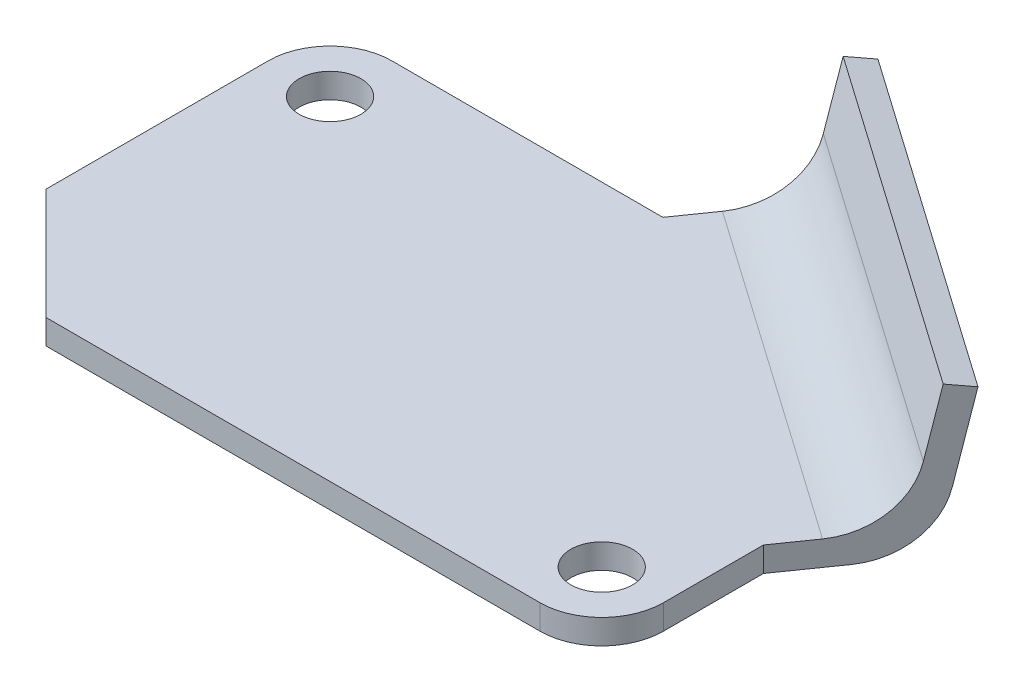
ISO-10303-21;
HEADER;
FILE_DESCRIPTION(('STEP AP214'),'2;1');
FILE_NAME('part.step','',(''),(''),'','','');
FILE_SCHEMA(('AUTOMOTIVE_DESIGN { 1 0 10303 214 1 1 1 1 }'));
ENDSEC;
DATA;
#1=APPLICATION_CONTEXT('core data for automotive mechanical design processes');
#2=APPLICATION_PROTOCOL_DEFINITION('international standard','automotive_design',2000,#1);
#3=PRODUCT_CONTEXT('',#1,'mechanical');
#4=PRODUCT('Part','Part','',(#3));
#5=PRODUCT_RELATED_PRODUCT_CATEGORY('part','',(#4));
#6=PRODUCT_DEFINITION_FORMATION('','',#4);
#7=PRODUCT_DEFINITION_CONTEXT('part definition',#1,'design');
#8=PRODUCT_DEFINITION('design','',#6,#7);
#9=PRODUCT_DEFINITION_SHAPE('','',#8);
#10=(LENGTH_UNIT() NAMED_UNIT(*) SI_UNIT(.MILLI.,.METRE.));
#11=(NAMED_UNIT(*) PLANE_ANGLE_UNIT() SI_UNIT($,.RADIAN.));
#12=(NAMED_UNIT(*) SI_UNIT($,.STERADIAN.) SOLID_ANGLE_UNIT());
#13=UNCERTAINTY_MEASURE_WITH_UNIT(LENGTH_MEASURE(1.E-05),#10,'distance_accuracy_value','');
#14=(GEOMETRIC_REPRESENTATION_CONTEXT(3) GLOBAL_UNCERTAINTY_ASSIGNED_CONTEXT((#13)) GLOBAL_UNIT_ASSIGNED_CONTEXT((#10,
#11,#12)) REPRESENTATION_CONTEXT('',''));
#15=CARTESIAN_POINT('',(0.,0.,0.));
#16=DIRECTION('',(0.,0.,1.));
#17=DIRECTION('',(1.,0.,0.));
#18=AXIS2_PLACEMENT_3D('',#15,#16,#17);
#19=CARTESIAN_POINT('',(0.,4.,-32.));
#20=DIRECTION('',(0.,0.,-1.));
#21=DIRECTION('',(-1.,0.,0.));
#22=AXIS2_PLACEMENT_3D('',#19,#20,#21);
#23=PLANE('',#22);
#24=DIRECTION('',(1.,0.,0.));
#25=VECTOR('',#24,1.);
#26=CARTESIAN_POINT('',(0.,0.,-32.));
#27=LINE('',#26,#25);
#28=CARTESIAN_POINT('',(-44.,0.,-32.));
#29=VERTEX_POINT('',#28);
#30=CARTESIAN_POINT('',(-0.0954306437080214,0.,-32.));
#31=VERTEX_POINT('',#30);
#32=EDGE_CURVE('E152',#29,#31,#27,.T.);
#33=ORIENTED_EDGE('',*,*,#32,.F.);
#34=DIRECTION('',(0.,-1.,0.));
#35=VECTOR('',#34,1.);
#36=CARTESIAN_POINT('',(-44.,4.,-32.));
#37=LINE('',#36,#35);
#38=CARTESIAN_POINT('',(-44.,4.,-32.));
#39=VERTEX_POINT('',#38);
#40=EDGE_CURVE('E241',#29,#39,#37,.F.);
#41=ORIENTED_EDGE('',*,*,#40,.T.);
#42=DIRECTION('',(1.,0.,0.));
#43=VECTOR('',#42,1.);
#44=CARTESIAN_POINT('',(0.,4.,-32.));
#45=LINE('',#44,#43);
#46=CARTESIAN_POINT('',(-0.0954306437080214,4.,-32.));
#47=VERTEX_POINT('',#46);
#48=EDGE_CURVE('E224',#39,#47,#45,.T.);
#49=ORIENTED_EDGE('',*,*,#48,.T.);
#50=DIRECTION('',(0.,-1.,0.));
#51=VECTOR('',#50,1.);
#52=CARTESIAN_POINT('',(-0.0954306437080294,4.,-32.));
#53=LINE('',#52,#51);
#54=EDGE_CURVE('E204',#47,#31,#53,.T.);
#55=ORIENTED_EDGE('',*,*,#54,.T.);
#56=EDGE_LOOP('',(#33,#41,#49,#55));
#57=FACE_BOUND('',#56,.T.);
#58=ADVANCED_FACE('F43',(#57),#23,.T.);
#59=CARTESIAN_POINT('',(0.,4.,0.));
#60=DIRECTION('',(0.,1.,0.));
#61=DIRECTION('',(0.,0.,1.));
#62=AXIS2_PLACEMENT_3D('',#59,#60,#61);
#63=PLANE('',#62);
#64=CARTESIAN_POINT('',(-44.,4.,-22.));
#65=DIRECTION('',(0.,1.,0.));
#66=DIRECTION('',(0.,0.,1.));
#67=AXIS2_PLACEMENT_3D('',#64,#65,#66);
#68=CIRCLE('',#67,5.);
#69=CARTESIAN_POINT('',(-44.,4.,-17.));
#70=VERTEX_POINT('',#69);
#71=EDGE_CURVE('E258',#70,#70,#68,.T.);
#72=ORIENTED_EDGE('',*,*,#71,.F.);
#73=EDGE_LOOP('',(#72));
#74=FACE_BOUND('',#73,.T.);
#75=CARTESIAN_POINT('',(44.,4.,22.));
#76=DIRECTION('',(0.,1.,0.));
#77=DIRECTION('',(0.,0.,1.));
#78=AXIS2_PLACEMENT_3D('',#75,#76,#77);
#79=CIRCLE('',#78,5.);
#80=CARTESIAN_POINT('',(44.,4.,27.));
#81=VERTEX_POINT('',#80);
#82=EDGE_CURVE('E263',#81,#81,#79,.T.);
#83=ORIENTED_EDGE('',*,*,#82,.F.);
#84=EDGE_LOOP('',(#83));
#85=FACE_BOUND('',#84,.T.);
#86=DIRECTION('',(0.,0.,-1.));
#87=VECTOR('',#86,1.);
#88=CARTESIAN_POINT('',(-54.,4.,0.));
#89=LINE('',#88,#87);
#90=CARTESIAN_POINT('',(-54.,4.,13.9999999999999));
#91=VERTEX_POINT('',#90);
#92=CARTESIAN_POINT('',(-54.,4.,-22.));
#93=VERTEX_POINT('',#92);
#94=EDGE_CURVE('E225',#91,#93,#89,.T.);
#95=ORIENTED_EDGE('',*,*,#94,.F.);
#96=DIRECTION('',(0.707106781186548,0.,0.707106781186548));
#97=VECTOR('',#96,1.);
#98=CARTESIAN_POINT('',(-34.,4.,34.));
#99=LINE('',#98,#97);
#100=CARTESIAN_POINT('',(-35.9999999999999,4.,32.));
#101=VERTEX_POINT('',#100);
#102=EDGE_CURVE('E11',#91,#101,#99,.T.);
#103=ORIENTED_EDGE('',*,*,#102,.T.);
#104=DIRECTION('',(1.,0.,0.));
#105=VECTOR('',#104,1.);
#106=CARTESIAN_POINT('',(0.,4.,32.));
#107=LINE('',#106,#105);
#108=CARTESIAN_POINT('',(44.,4.,32.));
#109=VERTEX_POINT('',#108);
#110=EDGE_CURVE('E217',#101,#109,#107,.T.);
#111=ORIENTED_EDGE('',*,*,#110,.T.);
#112=CARTESIAN_POINT('',(44.,4.,22.));
#113=DIRECTION('',(0.,1.,0.));
#114=DIRECTION('',(0.,0.,1.));
#115=AXIS2_PLACEMENT_3D('',#112,#113,#114);
#116=CIRCLE('',#115,10.);
#117=CARTESIAN_POINT('',(54.,4.,22.));
#118=VERTEX_POINT('',#117);
#119=EDGE_CURVE('E243',#109,#118,#116,.T.);
#120=ORIENTED_EDGE('',*,*,#119,.T.);
#121=DIRECTION('',(0.,0.,-1.));
#122=VECTOR('',#121,1.);
#123=CARTESIAN_POINT('',(54.,4.,0.));
#124=LINE('',#123,#122);
#125=CARTESIAN_POINT('',(54.,4.,5.81120706332445));
#126=VERTEX_POINT('',#125);
#127=EDGE_CURVE('E220',#118,#126,#124,.T.);
#128=ORIENTED_EDGE('',*,*,#127,.T.);
#129=DIRECTION('',(-0.573576436351047,0.,0.819152044288991));
#130=VECTOR('',#129,1.);
#131=CARTESIAN_POINT('',(59.7357643635105,4.,-2.38031337956546));
#132=LINE('',#131,#130);
#133=CARTESIAN_POINT('',(57.9434998164939,4.,0.17930566081089));
#134=VERTEX_POINT('',#133);
#135=EDGE_CURVE('E208',#134,#126,#132,.T.);
#136=ORIENTED_EDGE('',*,*,#135,.F.);
#137=DIRECTION('',(0.819152044288991,0.,0.573576436351048));
#138=VECTOR('',#137,1.);
#139=CARTESIAN_POINT('',(3.87946489342047,4.,-37.6767391383582));
#140=LINE('',#139,#138);
#141=CARTESIAN_POINT('',(3.87946489342047,4.,-37.6767391383582));
#142=VERTEX_POINT('',#141);
#143=EDGE_CURVE('E196',#142,#134,#140,.T.);
#144=ORIENTED_EDGE('',*,*,#143,.F.);
#145=DIRECTION('',(-0.573576436351048,0.,0.819152044288991));
#146=VECTOR('',#145,1.);
#147=CARTESIAN_POINT('',(-1.49365590296264,4.,-30.0031273830191));
#148=LINE('',#147,#146);
#149=EDGE_CURVE('E164',#142,#47,#148,.T.);
#150=ORIENTED_EDGE('',*,*,#149,.T.);
#151=ORIENTED_EDGE('',*,*,#48,.F.);
#152=CARTESIAN_POINT('',(-44.,4.,-22.));
#153=DIRECTION('',(0.,1.,0.));
#154=DIRECTION('',(0.,0.,1.));
#155=AXIS2_PLACEMENT_3D('',#152,#153,#154);
#156=CIRCLE('',#155,10.);
#157=EDGE_CURVE('E244',#39,#93,#156,.T.);
#158=ORIENTED_EDGE('',*,*,#157,.T.);
#159=EDGE_LOOP('',(#95,#103,#111,#120,#128,#136,#144,#150,#151,#158));
#160=FACE_BOUND('',#159,.T.);
#161=ADVANCED_FACE('F273',(#74,#85,#160),#63,.T.);
#162=CARTESIAN_POINT('',(0.,4.,32.));
#163=DIRECTION('',(0.,0.,-1.));
#164=DIRECTION('',(-1.,0.,0.));
#165=AXIS2_PLACEMENT_3D('',#162,#163,#164);
#166=PLANE('',#165);
#167=ORIENTED_EDGE('',*,*,#110,.F.);
#168=DIRECTION('',(0.,-1.,0.));
#169=VECTOR('',#168,1.);
#170=CARTESIAN_POINT('',(-35.9999999999999,0.,32.));
#171=LINE('',#170,#169);
#172=CARTESIAN_POINT('',(-35.9999999999999,0.,32.));
#173=VERTEX_POINT('',#172);
#174=EDGE_CURVE('E251',#101,#173,#171,.T.);
#175=ORIENTED_EDGE('',*,*,#174,.T.);
#176=DIRECTION('',(1.,0.,0.));
#177=VECTOR('',#176,1.);
#178=CARTESIAN_POINT('',(0.,0.,32.));
#179=LINE('',#178,#177);
#180=CARTESIAN_POINT('',(44.,0.,32.));
#181=VERTEX_POINT('',#180);
#182=EDGE_CURVE('E213',#173,#181,#179,.T.);
#183=ORIENTED_EDGE('',*,*,#182,.T.);
#184=DIRECTION('',(0.,-1.,0.));
#185=VECTOR('',#184,1.);
#186=CARTESIAN_POINT('',(44.,4.,32.));
#187=LINE('',#186,#185);
#188=EDGE_CURVE('E252',#181,#109,#187,.F.);
#189=ORIENTED_EDGE('',*,*,#188,.T.);
#190=EDGE_LOOP('',(#167,#175,#183,#189));
#191=FACE_BOUND('',#190,.T.);
#192=ADVANCED_FACE('F279',(#191),#166,.F.);
#193=CARTESIAN_POINT('',(54.,4.,0.));
#194=DIRECTION('',(-1.,0.,0.));
#195=DIRECTION('',(0.,0.,1.));
#196=AXIS2_PLACEMENT_3D('',#193,#194,#195);
#197=PLANE('',#196);
#198=ORIENTED_EDGE('',*,*,#127,.F.);
#199=DIRECTION('',(0.,-1.,0.));
#200=VECTOR('',#199,1.);
#201=CARTESIAN_POINT('',(54.,4.,22.));
#202=LINE('',#201,#200);
#203=CARTESIAN_POINT('',(54.,0.,22.));
#204=VERTEX_POINT('',#203);
#205=EDGE_CURVE('E247',#118,#204,#202,.T.);
#206=ORIENTED_EDGE('',*,*,#205,.T.);
#207=DIRECTION('',(0.,0.,-1.));
#208=VECTOR('',#207,1.);
#209=CARTESIAN_POINT('',(54.,0.,0.));
#210=LINE('',#209,#208);
#211=CARTESIAN_POINT('',(54.,0.,5.81120706332445));
#212=VERTEX_POINT('',#211);
#213=EDGE_CURVE('E227',#204,#212,#210,.T.);
#214=ORIENTED_EDGE('',*,*,#213,.T.);
#215=DIRECTION('',(0.,-1.,0.));
#216=VECTOR('',#215,1.);
#217=CARTESIAN_POINT('',(54.,4.,5.81120706332445));
#218=LINE('',#217,#216);
#219=EDGE_CURVE('E222',#126,#212,#218,.T.);
#220=ORIENTED_EDGE('',*,*,#219,.F.);
#221=EDGE_LOOP('',(#198,#206,#214,#220));
#222=FACE_BOUND('',#221,.T.);
#223=ADVANCED_FACE('F299',(#222),#197,.F.);
#224=CARTESIAN_POINT('',(-54.,4.,0.));
#225=DIRECTION('',(-1.,0.,0.));
#226=DIRECTION('',(0.,0.,1.));
#227=AXIS2_PLACEMENT_3D('',#224,#225,#226);
#228=PLANE('',#227);
#229=DIRECTION('',(0.,0.,-1.));
#230=VECTOR('',#229,1.);
#231=CARTESIAN_POINT('',(-54.,0.,0.));
#232=LINE('',#231,#230);
#233=CARTESIAN_POINT('',(-54.,0.,13.9999999999999));
#234=VERTEX_POINT('',#233);
#235=CARTESIAN_POINT('',(-54.,0.,-22.));
#236=VERTEX_POINT('',#235);
#237=EDGE_CURVE('E216',#234,#236,#232,.T.);
#238=ORIENTED_EDGE('',*,*,#237,.F.);
#239=DIRECTION('',(0.,1.,0.));
#240=VECTOR('',#239,1.);
#241=CARTESIAN_POINT('',(-54.,4.,13.9999999999999));
#242=LINE('',#241,#240);
#243=EDGE_CURVE('E52',#234,#91,#242,.T.);
#244=ORIENTED_EDGE('',*,*,#243,.T.);
#245=ORIENTED_EDGE('',*,*,#94,.T.);
#246=DIRECTION('',(0.,-1.,0.));
#247=VECTOR('',#246,1.);
#248=CARTESIAN_POINT('',(-54.,4.,-22.));
#249=LINE('',#248,#247);
#250=EDGE_CURVE('E231',#93,#236,#249,.T.);
#251=ORIENTED_EDGE('',*,*,#250,.T.);
#252=EDGE_LOOP('',(#238,#244,#245,#251));
#253=FACE_BOUND('',#252,.T.);
#254=ADVANCED_FACE('F312',(#253),#228,.T.);
#255=CARTESIAN_POINT('',(0.,0.,0.));
#256=DIRECTION('',(0.,1.,0.));
#257=DIRECTION('',(0.,0.,1.));
#258=AXIS2_PLACEMENT_3D('',#255,#256,#257);
#259=PLANE('',#258);
#260=CARTESIAN_POINT('',(-44.,0.,-22.));
#261=DIRECTION('',(0.,1.,0.));
#262=DIRECTION('',(0.,0.,1.));
#263=AXIS2_PLACEMENT_3D('',#260,#261,#262);
#264=CIRCLE('',#263,5.);
#265=CARTESIAN_POINT('',(-44.,0.,-17.));
#266=VERTEX_POINT('',#265);
#267=EDGE_CURVE('E48',#266,#266,#264,.T.);
#268=ORIENTED_EDGE('',*,*,#267,.T.);
#269=EDGE_LOOP('',(#268));
#270=FACE_BOUND('',#269,.T.);
#271=CARTESIAN_POINT('',(44.,0.,22.));
#272=DIRECTION('',(0.,1.,0.));
#273=DIRECTION('',(0.,0.,1.));
#274=AXIS2_PLACEMENT_3D('',#271,#272,#273);
#275=CIRCLE('',#274,5.);
#276=CARTESIAN_POINT('',(44.,0.,27.));
#277=VERTEX_POINT('',#276);
#278=EDGE_CURVE('E259',#277,#277,#275,.T.);
#279=ORIENTED_EDGE('',*,*,#278,.T.);
#280=EDGE_LOOP('',(#279));
#281=FACE_BOUND('',#280,.T.);
#282=ORIENTED_EDGE('',*,*,#182,.F.);
#283=DIRECTION('',(-0.707106781186548,0.,-0.707106781186548));
#284=VECTOR('',#283,1.);
#285=CARTESIAN_POINT('',(-35.9999999999999,0.,32.));
#286=LINE('',#285,#284);
#287=EDGE_CURVE('E70',#173,#234,#286,.T.);
#288=ORIENTED_EDGE('',*,*,#287,.T.);
#289=ORIENTED_EDGE('',*,*,#237,.T.);
#290=CARTESIAN_POINT('',(-44.,0.,-22.));
#291=DIRECTION('',(0.,1.,0.));
#292=DIRECTION('',(0.,0.,1.));
#293=AXIS2_PLACEMENT_3D('',#290,#291,#292);
#294=CIRCLE('',#293,10.);
#295=EDGE_CURVE('E237',#236,#29,#294,.F.);
#296=ORIENTED_EDGE('',*,*,#295,.T.);
#297=ORIENTED_EDGE('',*,*,#32,.T.);
#298=DIRECTION('',(0.573576436351047,0.,-0.819152044288991));
#299=VECTOR('',#298,1.);
#300=CARTESIAN_POINT('',(5.80984774414615,0.,-40.4336115588712));
#301=LINE('',#300,#299);
#302=CARTESIAN_POINT('',(5.80984774414615,0.,-40.4336115588712));
#303=VERTEX_POINT('',#302);
#304=EDGE_CURVE('E144',#31,#303,#301,.T.);
#305=ORIENTED_EDGE('',*,*,#304,.T.);
#306=DIRECTION('',(0.819152044288991,0.,0.573576436351048));
#307=VECTOR('',#306,1.);
#308=CARTESIAN_POINT('',(5.80984774414615,0.,-40.4336115588712));
#309=LINE('',#308,#307);
#310=CARTESIAN_POINT('',(59.8738826672195,0.,-2.57756675970206));
#311=VERTEX_POINT('',#310);
#312=EDGE_CURVE('E149',#303,#311,#309,.T.);
#313=ORIENTED_EDGE('',*,*,#312,.T.);
#314=DIRECTION('',(-0.573576436351047,0.,0.819152044288991));
#315=VECTOR('',#314,1.);
#316=CARTESIAN_POINT('',(59.7357643635105,0.,-2.38031337956546));
#317=LINE('',#316,#315);
#318=EDGE_CURVE('E214',#311,#212,#317,.T.);
#319=ORIENTED_EDGE('',*,*,#318,.T.);
#320=ORIENTED_EDGE('',*,*,#213,.F.);
#321=CARTESIAN_POINT('',(44.,0.,22.));
#322=DIRECTION('',(0.,1.,0.));
#323=DIRECTION('',(0.,0.,1.));
#324=AXIS2_PLACEMENT_3D('',#321,#322,#323);
#325=CIRCLE('',#324,10.);
#326=EDGE_CURVE('E236',#204,#181,#325,.F.);
#327=ORIENTED_EDGE('',*,*,#326,.T.);
#328=EDGE_LOOP('',(#282,#288,#289,#296,#297,#305,#313,#319,#320,#327));
#329=FACE_BOUND('',#328,.T.);
#330=ADVANCED_FACE('F147',(#270,#281,#329),#259,.F.);
#331=CARTESIAN_POINT('',(59.7357643635105,0.,-2.38031337956546));
#332=DIRECTION('',(-0.819152044288991,0.,-0.573576436351047));
#333=DIRECTION('',(-0.573576436351047,0.,0.819152044288991));
#334=AXIS2_PLACEMENT_3D('',#331,#332,#333);
#335=PLANE('',#334);
#336=CARTESIAN_POINT('',(57.9434998164939,16.,0.179305660810918));
#337=DIRECTION('',(-0.819152044288991,0.,-0.573576436351048));
#338=DIRECTION('',(0.573576436351048,0.,-0.819152044288991));
#339=AXIS2_PLACEMENT_3D('',#336,#337,#338);
#340=CIRCLE('',#339,12.);
#341=CARTESIAN_POINT('',(64.6682388612845,13.4421582791816,-9.42461700186756));
#342=VERTEX_POINT('',#341);
#343=EDGE_CURVE('E156',#342,#134,#340,.T.);
#344=ORIENTED_EDGE('',*,*,#343,.T.);
#345=ORIENTED_EDGE('',*,*,#135,.T.);
#346=ORIENTED_EDGE('',*,*,#219,.T.);
#347=ORIENTED_EDGE('',*,*,#318,.F.);
#348=CARTESIAN_POINT('',(59.8738826672196,12.,-2.57756675970213));
#349=DIRECTION('',(0.819152044288991,0.,0.573576436351048));
#350=DIRECTION('',(0.573576436351048,0.,-0.819152044288991));
#351=AXIS2_PLACEMENT_3D('',#348,#349,#350);
#352=CIRCLE('',#351,11.9999999999999);
#353=CARTESIAN_POINT('',(66.5986217120101,9.44215827918167,-12.1814894223806));
#354=VERTEX_POINT('',#353);
#355=EDGE_CURVE('E161',#311,#354,#352,.T.);
#356=ORIENTED_EDGE('',*,*,#355,.T.);
#357=DIRECTION('',(0.122259811581422,0.977018728252349,-0.174605106214672));
#358=VECTOR('',#357,1.);
#359=CARTESIAN_POINT('',(68.31025907415,23.1204204747146,-14.625960909386));
#360=LINE('',#359,#358);
#361=CARTESIAN_POINT('',(68.31025907415,23.1204204747146,-14.625960909386));
#362=VERTEX_POINT('',#361);
#363=EDGE_CURVE('E189',#354,#362,#360,.T.);
#364=ORIENTED_EDGE('',*,*,#363,.T.);
#365=DIRECTION('',(-0.560394920399217,0.213153476734867,0.800326888556541));
#366=VECTOR('',#365,1.);
#367=CARTESIAN_POINT('',(65.9897815164718,24.0030442121888,-11.311975510698));
#368=LINE('',#367,#366);
#369=CARTESIAN_POINT('',(65.9897815164718,24.0030442121888,-11.311975510698));
#370=VERTEX_POINT('',#369);
#371=EDGE_CURVE('E192',#362,#370,#368,.T.);
#372=ORIENTED_EDGE('',*,*,#371,.T.);
#373=DIRECTION('',(-0.122259811581421,-0.97701872825235,0.174605106214672));
#374=VECTOR('',#373,1.);
#375=CARTESIAN_POINT('',(64.6682388612844,13.4421582791816,-9.42461700186753));
#376=LINE('',#375,#374);
#377=EDGE_CURVE('E191',#370,#342,#376,.T.);
#378=ORIENTED_EDGE('',*,*,#377,.T.);
#379=EDGE_LOOP('',(#344,#345,#346,#347,#356,#364,#372,#378));
#380=FACE_BOUND('',#379,.T.);
#381=ADVANCED_FACE('F301',(#380),#335,.F.);
#382=CARTESIAN_POINT('',(3.87946489342051,16.,-37.6767391383582));
#383=DIRECTION('',(0.819152044288991,0.,0.573576436351048));
#384=DIRECTION('',(0.573576436351048,0.,-0.819152044288991));
#385=AXIS2_PLACEMENT_3D('',#382,#383,#384);
#386=CYLINDRICAL_SURFACE('',#385,12.);
#387=ORIENTED_EDGE('',*,*,#343,.F.);
#388=DIRECTION('',(0.819152044288991,0.,0.573576436351048));
#389=VECTOR('',#388,1.);
#390=CARTESIAN_POINT('',(10.6042039382111,13.4421582791816,-47.2806618010367));
#391=LINE('',#390,#389);
#392=CARTESIAN_POINT('',(10.6042039382111,13.4421582791816,-47.2806618010367));
#393=VERTEX_POINT('',#392);
#394=EDGE_CURVE('E201',#393,#342,#391,.T.);
#395=ORIENTED_EDGE('',*,*,#394,.F.);
#396=CARTESIAN_POINT('',(3.87946489342051,16.,-37.6767391383582));
#397=DIRECTION('',(-0.819152044288991,0.,-0.573576436351048));
#398=DIRECTION('',(0.573576436351048,0.,-0.819152044288991));
#399=AXIS2_PLACEMENT_3D('',#396,#397,#398);
#400=CIRCLE('',#399,12.);
#401=EDGE_CURVE('E185',#393,#142,#400,.T.);
#402=ORIENTED_EDGE('',*,*,#401,.T.);
#403=ORIENTED_EDGE('',*,*,#143,.T.);
#404=EDGE_LOOP('',(#387,#395,#402,#403));
#405=FACE_BOUND('',#404,.T.);
#406=ADVANCED_FACE('F306',(#405),#386,.F.);
#407=CARTESIAN_POINT('',(10.6042039382111,13.4421582791816,-47.2806618010367));
#408=DIRECTION('',(-0.560394920399215,0.213153476734867,0.800326888556542));
#409=DIRECTION('',(0.819152044288991,0.,0.573576436351048));
#410=AXIS2_PLACEMENT_3D('',#407,#408,#409);
#411=PLANE('',#410);
#412=ORIENTED_EDGE('',*,*,#377,.F.);
#413=DIRECTION('',(0.819152044288991,0.,0.573576436351048));
#414=VECTOR('',#413,1.);
#415=CARTESIAN_POINT('',(11.9257465933984,24.0030442121888,-49.1680203098671));
#416=LINE('',#415,#414);
#417=CARTESIAN_POINT('',(11.9257465933984,24.0030442121888,-49.1680203098671));
#418=VERTEX_POINT('',#417);
#419=EDGE_CURVE('E203',#418,#370,#416,.T.);
#420=ORIENTED_EDGE('',*,*,#419,.F.);
#421=DIRECTION('',(-0.122259811581421,-0.97701872825235,0.174605106214672));
#422=VECTOR('',#421,1.);
#423=CARTESIAN_POINT('',(10.6042039382111,13.4421582791816,-47.2806618010367));
#424=LINE('',#423,#422);
#425=EDGE_CURVE('E177',#418,#393,#424,.T.);
#426=ORIENTED_EDGE('',*,*,#425,.T.);
#427=ORIENTED_EDGE('',*,*,#394,.T.);
#428=EDGE_LOOP('',(#412,#420,#426,#427));
#429=FACE_BOUND('',#428,.T.);
#430=ADVANCED_FACE('F346',(#429),#411,.T.);
#431=CARTESIAN_POINT('',(11.9257465933984,24.0030442121888,-49.1680203098671));
#432=DIRECTION('',(0.122259811581421,0.977018728252349,-0.174605106214672));
#433=DIRECTION('',(0.,0.175924871694795,0.984403595848354));
#434=AXIS2_PLACEMENT_3D('',#431,#432,#433);
#435=PLANE('',#434);
#436=ORIENTED_EDGE('',*,*,#371,.F.);
#437=DIRECTION('',(0.819152044288991,0.,0.573576436351048));
#438=VECTOR('',#437,1.);
#439=CARTESIAN_POINT('',(14.2462241510766,23.1204204747146,-52.4820057085551));
#440=LINE('',#439,#438);
#441=CARTESIAN_POINT('',(14.2462241510766,23.1204204747146,-52.4820057085551));
#442=VERTEX_POINT('',#441);
#443=EDGE_CURVE('E207',#442,#362,#440,.T.);
#444=ORIENTED_EDGE('',*,*,#443,.F.);
#445=DIRECTION('',(-0.560394920399217,0.213153476734867,0.800326888556541));
#446=VECTOR('',#445,1.);
#447=CARTESIAN_POINT('',(11.9257465933984,24.0030442121888,-49.1680203098671));
#448=LINE('',#447,#446);
#449=EDGE_CURVE('E173',#442,#418,#448,.T.);
#450=ORIENTED_EDGE('',*,*,#449,.T.);
#451=ORIENTED_EDGE('',*,*,#419,.T.);
#452=EDGE_LOOP('',(#436,#444,#450,#451));
#453=FACE_BOUND('',#452,.T.);
#454=ADVANCED_FACE('F351',(#453),#435,.T.);
#455=CARTESIAN_POINT('',(14.2462241510766,23.1204204747146,-52.4820057085551));
#456=DIRECTION('',(0.560394920399215,-0.213153476734867,-0.800326888556542));
#457=DIRECTION('',(-0.819152044288991,0.,-0.573576436351048));
#458=AXIS2_PLACEMENT_3D('',#455,#456,#457);
#459=PLANE('',#458);
#460=ORIENTED_EDGE('',*,*,#363,.F.);
#461=DIRECTION('',(0.819152044288991,0.,0.573576436351048));
#462=VECTOR('',#461,1.);
#463=CARTESIAN_POINT('',(12.5345867889367,9.44215827918167,-50.0375342215497));
#464=LINE('',#463,#462);
#465=CARTESIAN_POINT('',(12.5345867889367,9.44215827918167,-50.0375342215497));
#466=VERTEX_POINT('',#465);
#467=EDGE_CURVE('E165',#466,#354,#464,.T.);
#468=ORIENTED_EDGE('',*,*,#467,.F.);
#469=DIRECTION('',(0.122259811581422,0.977018728252349,-0.174605106214672));
#470=VECTOR('',#469,1.);
#471=CARTESIAN_POINT('',(14.2462241510766,23.1204204747146,-52.4820057085551));
#472=LINE('',#471,#470);
#473=EDGE_CURVE('E171',#466,#442,#472,.T.);
#474=ORIENTED_EDGE('',*,*,#473,.T.);
#475=ORIENTED_EDGE('',*,*,#443,.T.);
#476=EDGE_LOOP('',(#460,#468,#474,#475));
#477=FACE_BOUND('',#476,.T.);
#478=ADVANCED_FACE('F358',(#477),#459,.T.);
#479=CARTESIAN_POINT('',(5.8098477441462,12.,-40.4336115588713));
#480=DIRECTION('',(0.819152044288991,0.,0.573576436351048));
#481=DIRECTION('',(0.573576436351048,0.,-0.819152044288991));
#482=AXIS2_PLACEMENT_3D('',#479,#480,#481);
#483=CYLINDRICAL_SURFACE('',#482,11.9999999999999);
#484=ORIENTED_EDGE('',*,*,#355,.F.);
#485=ORIENTED_EDGE('',*,*,#312,.F.);
#486=CARTESIAN_POINT('',(5.8098477441462,12.,-40.4336115588713));
#487=DIRECTION('',(0.819152044288991,0.,0.573576436351048));
#488=DIRECTION('',(0.573576436351048,0.,-0.819152044288991));
#489=AXIS2_PLACEMENT_3D('',#486,#487,#488);
#490=CIRCLE('',#489,11.9999999999999);
#491=EDGE_CURVE('E159',#303,#466,#490,.T.);
#492=ORIENTED_EDGE('',*,*,#491,.T.);
#493=ORIENTED_EDGE('',*,*,#467,.T.);
#494=EDGE_LOOP('',(#484,#485,#492,#493));
#495=FACE_BOUND('',#494,.T.);
#496=ADVANCED_FACE('F163',(#495),#483,.T.);
#497=CARTESIAN_POINT('',(3.87946489342051,16.,-37.6767391383582));
#498=DIRECTION('',(0.819152044288991,0.,0.573576436351048));
#499=DIRECTION('',(0.573576436351048,0.,-0.819152044288991));
#500=AXIS2_PLACEMENT_3D('',#497,#498,#499);
#501=PLANE('',#500);
#502=ORIENTED_EDGE('',*,*,#54,.F.);
#503=ORIENTED_EDGE('',*,*,#149,.F.);
#504=ORIENTED_EDGE('',*,*,#401,.F.);
#505=ORIENTED_EDGE('',*,*,#425,.F.);
#506=ORIENTED_EDGE('',*,*,#449,.F.);
#507=ORIENTED_EDGE('',*,*,#473,.F.);
#508=ORIENTED_EDGE('',*,*,#491,.F.);
#509=ORIENTED_EDGE('',*,*,#304,.F.);
#510=EDGE_LOOP('',(#502,#503,#504,#505,#506,#507,#508,#509));
#511=FACE_BOUND('',#510,.T.);
#512=ADVANCED_FACE('F166',(#511),#501,.F.);
#513=CARTESIAN_POINT('',(-44.,4.,-22.));
#514=DIRECTION('',(0.,-1.,0.));
#515=DIRECTION('',(0.,0.,-1.));
#516=AXIS2_PLACEMENT_3D('',#513,#514,#515);
#517=CYLINDRICAL_SURFACE('',#516,10.);
#518=ORIENTED_EDGE('',*,*,#157,.F.);
#519=ORIENTED_EDGE('',*,*,#40,.F.);
#520=ORIENTED_EDGE('',*,*,#295,.F.);
#521=ORIENTED_EDGE('',*,*,#250,.F.);
#522=EDGE_LOOP('',(#518,#519,#520,#521));
#523=FACE_BOUND('',#522,.T.);
#524=ADVANCED_FACE('F311',(#523),#517,.T.);
#525=CARTESIAN_POINT('',(44.,4.,22.));
#526=DIRECTION('',(0.,-1.,0.));
#527=DIRECTION('',(0.,0.,-1.));
#528=AXIS2_PLACEMENT_3D('',#525,#526,#527);
#529=CYLINDRICAL_SURFACE('',#528,10.);
#530=ORIENTED_EDGE('',*,*,#119,.F.);
#531=ORIENTED_EDGE('',*,*,#188,.F.);
#532=ORIENTED_EDGE('',*,*,#326,.F.);
#533=ORIENTED_EDGE('',*,*,#205,.F.);
#534=EDGE_LOOP('',(#530,#531,#532,#533));
#535=FACE_BOUND('',#534,.T.);
#536=ADVANCED_FACE('F295',(#535),#529,.T.);
#537=CARTESIAN_POINT('',(-35.9999999999999,4.,32.));
#538=DIRECTION('',(-0.707106781186547,0.,0.707106781186547));
#539=DIRECTION('',(0.,1.,0.));
#540=AXIS2_PLACEMENT_3D('',#537,#538,#539);
#541=PLANE('',#540);
#542=ORIENTED_EDGE('',*,*,#102,.F.);
#543=ORIENTED_EDGE('',*,*,#243,.F.);
#544=ORIENTED_EDGE('',*,*,#287,.F.);
#545=ORIENTED_EDGE('',*,*,#174,.F.);
#546=EDGE_LOOP('',(#542,#543,#544,#545));
#547=FACE_BOUND('',#546,.T.);
#548=ADVANCED_FACE('F46',(#547),#541,.T.);
#549=CARTESIAN_POINT('',(44.,-62.,22.));
#550=DIRECTION('',(0.,1.,0.));
#551=DIRECTION('',(0.,0.,1.));
#552=AXIS2_PLACEMENT_3D('',#549,#550,#551);
#553=CYLINDRICAL_SURFACE('',#552,5.);
#554=ORIENTED_EDGE('',*,*,#82,.T.);
#555=EDGE_LOOP('',(#554));
#556=FACE_BOUND('',#555,.T.);
#557=ORIENTED_EDGE('',*,*,#278,.F.);
#558=EDGE_LOOP('',(#557));
#559=FACE_BOUND('',#558,.T.);
#560=ADVANCED_FACE('F275',(#556,#559),#553,.F.);
#561=CARTESIAN_POINT('',(-44.,-62.,-22.));
#562=DIRECTION('',(0.,1.,0.));
#563=DIRECTION('',(0.,0.,1.));
#564=AXIS2_PLACEMENT_3D('',#561,#562,#563);
#565=CYLINDRICAL_SURFACE('',#564,5.);
#566=ORIENTED_EDGE('',*,*,#71,.T.);
#567=EDGE_LOOP('',(#566));
#568=FACE_BOUND('',#567,.T.);
#569=ORIENTED_EDGE('',*,*,#267,.F.);
#570=EDGE_LOOP('',(#569));
#571=FACE_BOUND('',#570,.T.);
#572=ADVANCED_FACE('F339',(#568,#571),#565,.F.);
#573=CLOSED_SHELL('',(#58,#161,#192,#223,#254,#330,#381,#406,#430,#454,#478,#496,#512,#524,#536,
#548,#560,#572));
#574=MANIFOLD_SOLID_BREP('B2',#573);
#575=ADVANCED_BREP_SHAPE_REPRESENTATION('',(#18,#574),#14);
#576=SHAPE_DEFINITION_REPRESENTATION(#9,#575);
ENDSEC;
END-ISO-10303-21;
